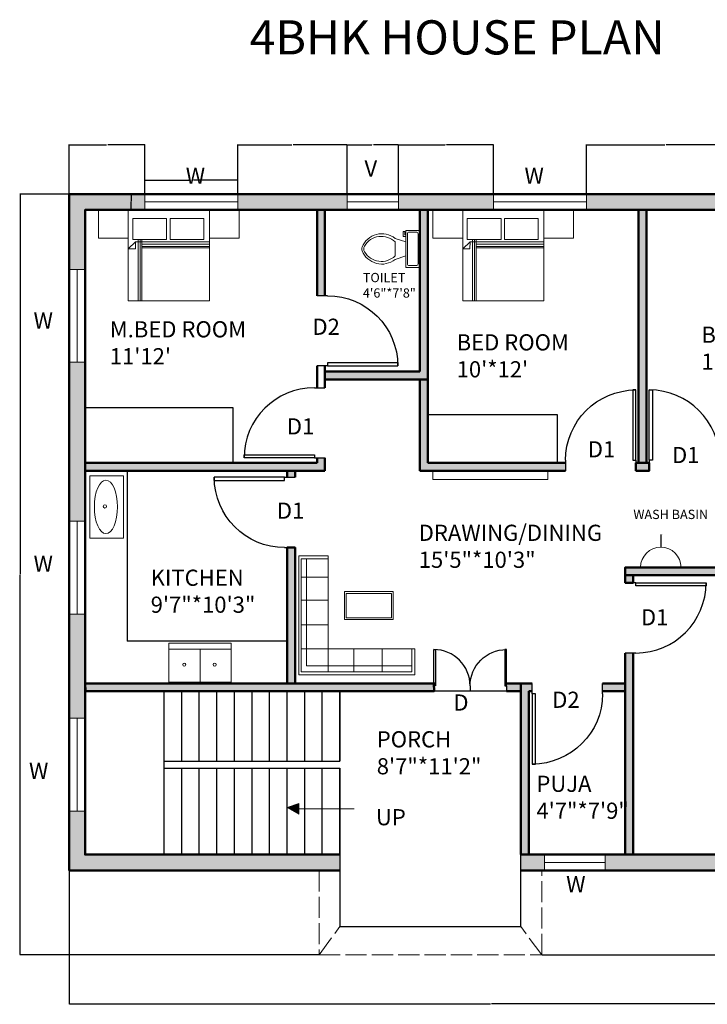
# Model space of a CAD drawing. Units: inches. Extents: x 2116 to 2704, y 2001 to 2561.
# Tile 1 of 2: x 2116 to 2508, y 2001 to 2561. Entities that reach past the tile are written whole.
import ezdxf

# ---------------------------------------------------------------- set-up
doc = ezdxf.new("R2010")
doc.units = ezdxf.units.IN
doc.linetypes.add('ACAD_ISO02W100', pattern=[15, 12, -3])
for name, color, linetype, lineweight in [('A-ANNO-DIMS', 2, 'Continuous', 18), ('A-ANNO-SYMB', 70, 'Continuous', 18), ('A-ANNO-TITL', 7, 'Continuous', 35), ('A-AREA-IDEN', 70, 'Continuous', 25), ('A-DOOR', 3, 'Continuous', 25), ('A-FLOR', 7, 'Continuous', 30), ('A-FLOR-CASE', 9, 'Continuous', 25), ('A-FLOR-FIXT', 9, 'Continuous', 18), ('A-FLOR-OVHD', 8, 'ACAD_ISO02W100', 18), ('A-FLOR-STRS', 7, 'Continuous', 25), ('A-FURN', 40, 'Continuous', 18), ('A-GLAZ', 4, 'Continuous', 20), ('A-WALL-PATT', 172, 'Continuous', 13), ('SINK', 240, 'Continuous', 18), ('TEXT', 70, 'Continuous', 18), ('TV', 210, 'Continuous', 18), ('WALL', 7, 'Continuous', 50)]:
    doc.layers.add(name, color=color, linetype=linetype, lineweight=lineweight)
doc.styles.get("Standard").update_dxf_attribs({"font": 'arial.ttf'})
doc.dimstyles.get("Standard").update_dxf_attribs({"dimtxt": 0.18, "dimasz": 0.18, "dimexe": 0.18, "dimexo": 0.0625, "dimgap": 0.09, "dimtad": 0, "dimtih": 1, "dimtoh": 1, "dimdec": 4, "dimzin": 0, "dimdsep": 46, "dimtxsty": 'Standard', "dimcen": 0.09, "dimadec": 0, "dimazin": 0, "dimtfac": 1, "dimtdec": 4, "dimtofl": 0, "dimtmove": 0, "dimatfit": 3, "dimfxl": 1, "dimtolj": 1, "dimtzin": 0, "dimarcsym": 0})

# ---------------------------------------------------------------- blocks, each defined once
blk = doc.blocks.new('*U2')
for p, q in [((0, 0), (0, -6)), ((40, 0), (40, -6))]:
    blk.add_line(p, q)
blk.add_lwpolyline([(0, 0), (0, 40), (1.75, 40), (1.75, 0)], close=True)
blk.add_arc((0, 0), 40, 0, 90)
blk = doc.blocks.new('*U4')
for p, q in [((9.5, -6), (9.5, -2)), ((-10, -8.5), (-8, -8.5)), ((-10, -9.5), (-10, -8.5)), ((-7, -9.5), (-10, -9.5)), ((-8, -8.5), (-8, -8)), ((-7, -8), (-7, -9.5)), ((-4, -8), (-6, -14)), ((4, -8), (6, -14)), ((4, -14), (-4, -14))]:
    blk.add_line(p, q)
blk.add_lwpolyline([(10.5, -8), (10.5, 0), (-10.5, 0), (-10.5, -8)], close=True)
for points in [[(-9.5, -2), (-9.5, -6)], [(8.5, -1), (-8.5, -1)], [(-8.5, -7), (8.5, -7)]]:
    blk.add_lwpolyline(points)
for centre, radius, start, end in [((-8.62, -1.88), 0.884, 81.8699, 188.1301), ((8.62, -1.88), 0.884, 351.8699, 98.1301), ((-8.62, -6.12), 0.884, 171.8699, 278.1301), ((8.62, -6.12), 0.884, 261.8699, 8.1301), ((3.52, -21.58), 12.17, 141.4691, 247.9714), ((4.2, -21.82), 11.33, 136.3677, 238.9468), ((-3.52, -21.58), 12.17, 292.0284, 38.5307), ((-4.2, -21.82), 11.33, 301.053, 43.6321), ((0, -27.88), 4, 245.7318, 294.2682), ((0, -29), 4, 254.8605, 285.1395)]:
    blk.add_arc(centre, radius, start, end)
blk = doc.blocks.new('BED-DOUBLE-WITH-NIGHTSTANDS')
for p, q in [((22.66, 34.94), (22.66, 0)), ((23.77, 34.94), (23.77, 0)), ((24.74, 34.94), (24.74, 0)), ((21.16, 33.51), (16.99, 29.58)), ((16.99, 29.58), (21.04, 29.58)), ((21.04, 29.58), (21.16, 33.51)), ((63.16, 33.51), (21.16, 33.51)), ((24.74, 32.21), (63.16, 32.21)), ((24.74, 30.97), (63.16, 30.97)), ((24.74, 30.05), (63.16, 30.05))]:
    blk.add_line(p, q)
for points in [[(16.99, 51.74), (0, 51.74), (0, 35.55), (16.99, 35.55)], [(16.99, 51.74), (63.16, 51.74), (63.16, 0), (16.99, 0)], [(80.15, 51.74), (63.16, 51.74), (63.16, 35.55), (80.15, 35.55)], [(19.62, 46.86), (38.84, 46.86), (38.84, 34.94), (19.62, 34.94)], [(40.77, 46.86), (59.99, 46.86), (59.99, 34.94), (40.77, 34.94)]]:
    blk.add_lwpolyline(points, close=True)
blk = doc.blocks.new('WIN-PLAN-53IN-NOM')
blk.add_line((0, 4.5), (52.88, 4.5))
blk.add_lwpolyline([(0, 9), (52.88, 9), (52.88, 0), (0, 0)], close=True)
blk = doc.blocks.new('*D7')
at = {"layer": 'A-ANNO-DIMS', "color": 0, "lineweight": -2, "transparency": 16777216}
for p, q in [((2187.79, 2462.31), (2187.79, 2470.36)), ((2187.97, 2470.18), (2213.11, 2470.18)), ((2240.48, 2470.18), (2215.34, 2470.18)), ((2240.66, 2462.31), (2240.66, 2470.36))]:
    blk.add_line(p, q, dxfattribs=at)
at = {"layer": 'A-ANNO-DIMS', "color": 0, "lineweight": 100, "transparency": 16777216}
for points in [[(2187.97, 2470.21), (2187.97, 2470.15), (2187.79, 2470.18)], [(2240.48, 2470.21), (2240.48, 2470.15), (2240.66, 2470.18)]]:
    blk.add_solid(points, dxfattribs=at)
at = {"layer": 'Defpoints', "color": 0, "lineweight": 100, "transparency": 16777216}
for p in [(2240.66, 2470.18), (2187.79, 2462.24), (2240.66, 2462.24)]:
    blk.add_point(p, dxfattribs=at)
at = {"layer": 'A-ANNO-DIMS', "color": 0, "transparency": 16777216, "insert": (2214.22, 2470.18), "char_height": 0.18, "attachment_point": 5}
blk.add_mtext('\\A1;WINDOW 53 TYP.', dxfattribs=at)
blk = doc.blocks.new('*D8')
at = {"layer": 'A-ANNO-DIMS', "color": 0, "lineweight": -2, "transparency": 16777216}
for p, q in [((2187.72, 2462.24), (2179.67, 2462.24)), ((2179.85, 2462.06), (2179.85, 2457.93)), ((2179.85, 2453.42), (2179.85, 2457.56)), ((2187.72, 2453.24), (2179.67, 2453.24))]:
    blk.add_line(p, q, dxfattribs=at)
at = {"layer": 'A-ANNO-DIMS', "color": 0, "lineweight": 100, "transparency": 16777216}
for points in [[(2179.82, 2462.06), (2179.88, 2462.06), (2179.85, 2462.24)], [(2179.82, 2453.42), (2179.88, 2453.42), (2179.85, 2453.24)]]:
    blk.add_solid(points, dxfattribs=at)
at = {"layer": 'Defpoints', "color": 0, "lineweight": 100, "transparency": 16777216}
for p in [(2179.85, 2462.24), (2187.79, 2462.24), (2187.79, 2453.24)]:
    blk.add_point(p, dxfattribs=at)
at = {"layer": 'A-ANNO-DIMS', "color": 0, "transparency": 16777216, "insert": (2179.85, 2457.74), "char_height": 0.18, "attachment_point": 5}
blk.add_mtext('\\A1;9 TYP.', dxfattribs=at)
blk = doc.blocks.new('*D11')
at = {"layer": 'A-ANNO-DIMS', "color": 0, "lineweight": -2, "transparency": 16777216}
for p, q in [((2144.72, 2462.31), (2144.72, 2490.37)), ((2144.9, 2490.19), (2165.86, 2490.19)), ((2187.61, 2490.19), (2166.65, 2490.19)), ((2187.79, 2462.31), (2187.79, 2490.37))]:
    blk.add_line(p, q, dxfattribs=at)
at = {"layer": 'A-ANNO-DIMS', "color": 0, "lineweight": 100, "transparency": 16777216}
for points in [[(2144.9, 2490.22), (2144.9, 2490.16), (2144.72, 2490.19)], [(2187.61, 2490.22), (2187.61, 2490.16), (2187.79, 2490.19)]]:
    blk.add_solid(points, dxfattribs=at)
at = {"layer": 'Defpoints', "color": 0, "lineweight": 100, "transparency": 16777216}
for p in [(2187.79, 2490.19), (2144.72, 2462.24), (2187.79, 2462.24)]:
    blk.add_point(p, dxfattribs=at)
at = {"layer": 'A-ANNO-DIMS', "color": 0, "transparency": 16777216, "insert": (2166.25, 2490.19), "char_height": 0.18, "attachment_point": 5}
blk.add_mtext('\\A1;43.06', dxfattribs=at)
blk = doc.blocks.new('*D12')
at = {"layer": 'A-ANNO-DIMS', "color": 0, "lineweight": -2, "transparency": 16777216}
for p, q in [((2240.66, 2462.31), (2240.66, 2490.37)), ((2240.84, 2490.19), (2271.39, 2490.19)), ((2302.73, 2490.19), (2272.18, 2490.19)), ((2302.91, 2462.31), (2302.91, 2490.37))]:
    blk.add_line(p, q, dxfattribs=at)
at = {"layer": 'A-ANNO-DIMS', "color": 0, "lineweight": 100, "transparency": 16777216}
for points in [[(2240.84, 2490.22), (2240.84, 2490.16), (2240.66, 2490.19)], [(2302.73, 2490.22), (2302.73, 2490.16), (2302.91, 2490.19)]]:
    blk.add_solid(points, dxfattribs=at)
at = {"layer": 'Defpoints', "color": 0, "lineweight": 100, "transparency": 16777216}
for p in [(2302.91, 2490.19), (2240.66, 2462.24), (2302.91, 2462.24)]:
    blk.add_point(p, dxfattribs=at)
at = {"layer": 'A-ANNO-DIMS', "color": 0, "transparency": 16777216, "insert": (2271.79, 2490.19), "char_height": 0.18, "attachment_point": 5}
blk.add_mtext('\\A1;62.25', dxfattribs=at)
blk = doc.blocks.new('*D13')
at = {"layer": 'A-ANNO-DIMS', "color": 0, "lineweight": -2, "transparency": 16777216}
for p, q in [((2302.91, 2462.31), (2302.91, 2490.37)), ((2303.09, 2490.19), (2317.01, 2490.19)), ((2331.86, 2490.19), (2317.94, 2490.19)), ((2332.04, 2462.31), (2332.04, 2490.37))]:
    blk.add_line(p, q, dxfattribs=at)
at = {"layer": 'A-ANNO-DIMS', "color": 0, "lineweight": 100, "transparency": 16777216}
for points in [[(2303.09, 2490.22), (2303.09, 2490.16), (2302.91, 2490.19)], [(2331.86, 2490.22), (2331.86, 2490.16), (2332.04, 2490.19)]]:
    blk.add_solid(points, dxfattribs=at)
at = {"layer": 'Defpoints', "color": 0, "lineweight": 100, "transparency": 16777216}
for p in [(2332.04, 2490.19), (2302.91, 2462.24), (2332.04, 2462.24)]:
    blk.add_point(p, dxfattribs=at)
at = {"layer": 'A-ANNO-DIMS', "color": 0, "transparency": 16777216, "insert": (2317.47, 2490.19), "char_height": 0.18, "attachment_point": 5}
blk.add_mtext('\\A1;29.126', dxfattribs=at)
blk = doc.blocks.new('*D14')
at = {"layer": 'A-ANNO-DIMS', "color": 0, "lineweight": -2, "transparency": 16777216}
for p, q in [((2332.04, 2462.31), (2332.04, 2490.37)), ((2332.22, 2490.19), (2358.74, 2490.19)), ((2386.04, 2490.19), (2359.52, 2490.19)), ((2386.22, 2462.31), (2386.22, 2490.37))]:
    blk.add_line(p, q, dxfattribs=at)
at = {"layer": 'A-ANNO-DIMS', "color": 0, "lineweight": 100, "transparency": 16777216}
for points in [[(2332.22, 2490.22), (2332.22, 2490.16), (2332.04, 2490.19)], [(2386.04, 2490.22), (2386.04, 2490.16), (2386.22, 2490.19)]]:
    blk.add_solid(points, dxfattribs=at)
at = {"layer": 'Defpoints', "color": 0, "lineweight": 100, "transparency": 16777216}
for p in [(2386.22, 2490.19), (2332.04, 2462.24), (2386.22, 2462.24)]:
    blk.add_point(p, dxfattribs=at)
at = {"layer": 'A-ANNO-DIMS', "color": 0, "transparency": 16777216, "insert": (2359.13, 2490.19), "char_height": 0.18, "attachment_point": 5}
blk.add_mtext('\\A1;54.18', dxfattribs=at)
blk = doc.blocks.new('*D15')
at = {"layer": 'A-ANNO-DIMS', "color": 0, "lineweight": -2, "transparency": 16777216}
for p, q in [((2439.1, 2462.31), (2439.1, 2490.37)), ((2439.28, 2490.19), (2483.65, 2490.19)), ((2528.8, 2490.19), (2484.43, 2490.19)), ((2528.98, 2462.31), (2528.98, 2490.37))]:
    blk.add_line(p, q, dxfattribs=at)
at = {"layer": 'A-ANNO-DIMS', "color": 0, "lineweight": 100, "transparency": 16777216}
for points in [[(2439.28, 2490.22), (2439.28, 2490.16), (2439.1, 2490.19)], [(2528.8, 2490.22), (2528.8, 2490.16), (2528.98, 2490.19)]]:
    blk.add_solid(points, dxfattribs=at)
at = {"layer": 'Defpoints', "color": 0, "lineweight": 100, "transparency": 16777216}
for p in [(2528.98, 2490.19), (2439.1, 2462.24), (2528.98, 2462.24)]:
    blk.add_point(p, dxfattribs=at)
at = {"layer": 'A-ANNO-DIMS', "color": 0, "transparency": 16777216, "insert": (2484.04, 2490.19), "char_height": 0.18, "attachment_point": 5}
blk.add_mtext('\\A1;89.88', dxfattribs=at)
blk = doc.blocks.new('*D16')
at = {"layer": 'A-ANNO-DIMS', "color": 0, "lineweight": -2, "transparency": 16777216}
for p, q in [((2144.72, 2077.18), (2144.72, 2001.04)), ((2624.72, 2077.18), (2624.72, 2001.04)), ((2144.9, 2001.22), (2384.43, 2001.22)), ((2624.54, 2001.22), (2385.01, 2001.22))]:
    blk.add_line(p, q, dxfattribs=at)
at = {"layer": 'A-ANNO-DIMS', "color": 0, "lineweight": 100, "transparency": 16777216}
for points in [[(2144.9, 2001.25), (2144.9, 2001.19), (2144.72, 2001.22)], [(2624.54, 2001.25), (2624.54, 2001.19), (2624.72, 2001.22)]]:
    blk.add_solid(points, dxfattribs=at)
at = {"layer": 'Defpoints', "color": 0, "lineweight": 100, "transparency": 16777216}
for p in [(2144.72, 2077.24), (2624.72, 2077.24), (2624.72, 2001.22)]:
    blk.add_point(p, dxfattribs=at)
at = {"layer": 'A-ANNO-DIMS', "color": 0, "transparency": 16777216, "insert": (2384.72, 2001.22), "char_height": 0.18, "attachment_point": 5}
blk.add_mtext('\\A1;480', dxfattribs=at)
blk = doc.blocks.new('*D21')
at = {"layer": 'A-ANNO-DIMS', "color": 0, "lineweight": -2, "transparency": 16777216}
for p, q in [((2624.78, 2077.24), (2703.85, 2077.24)), ((2703.67, 2077.06), (2703.67, 2053.39)), ((2703.67, 2029.35), (2703.67, 2053.03)), ((2413.8, 2029.17), (2703.85, 2029.17))]:
    blk.add_line(p, q, dxfattribs=at)
at = {"layer": 'A-ANNO-DIMS', "color": 0, "lineweight": 100, "transparency": 16777216}
for points in [[(2703.64, 2077.06), (2703.7, 2077.06), (2703.67, 2077.24)], [(2703.64, 2029.35), (2703.7, 2029.35), (2703.67, 2029.17)]]:
    blk.add_solid(points, dxfattribs=at)
at = {"layer": 'Defpoints', "color": 0, "lineweight": 100, "transparency": 16777216}
for p in [(2624.72, 2077.24), (2703.67, 2077.24), (2413.74, 2029.17)]:
    blk.add_point(p, dxfattribs=at)
at = {"layer": 'A-ANNO-DIMS', "color": 0, "transparency": 16777216, "insert": (2703.67, 2053.21), "char_height": 0.18, "attachment_point": 5}
blk.add_mtext('\\A1;48.07', dxfattribs=at)
blk = doc.blocks.new('*D22')
at = {"layer": 'A-ANNO-DIMS', "color": 0, "lineweight": -2, "transparency": 16777216}
for p, q in [((2144.66, 2462.24), (2116.59, 2462.24)), ((2116.77, 2462.06), (2116.77, 2245.89)), ((2116.77, 2029.35), (2116.77, 2245.53)), ((2286.92, 2029.17), (2116.59, 2029.17))]:
    blk.add_line(p, q, dxfattribs=at)
at = {"layer": 'A-ANNO-DIMS', "color": 0, "lineweight": 100, "transparency": 16777216}
for points in [[(2116.74, 2462.06), (2116.8, 2462.06), (2116.77, 2462.24)], [(2116.74, 2029.35), (2116.8, 2029.35), (2116.77, 2029.17)]]:
    blk.add_solid(points, dxfattribs=at)
at = {"layer": 'Defpoints', "color": 0, "lineweight": 100, "transparency": 16777216}
for p in [(2116.77, 2462.24), (2144.72, 2462.24), (2286.98, 2029.17)]:
    blk.add_point(p, dxfattribs=at)
at = {"layer": 'A-ANNO-DIMS', "color": 0, "transparency": 16777216, "insert": (2116.77, 2245.71), "char_height": 0.18, "attachment_point": 5}
blk.add_mtext('\\A1;433.1', dxfattribs=at)
blk = doc.blocks.new('*D23')
at = {"layer": 'A-ANNO-DIMS', "color": 0, "lineweight": -2, "transparency": 16777216}
for p, q in [((2481.6, 2268.18), (2481.42, 2268.18)), ((2481.42, 2268.18), (2481.42, 2261.45)), ((2481.33, 2249.74), (2481.51, 2249.74)), ((2481.42, 2249.65), (2481.42, 2249.83))]:
    blk.add_line(p, q, dxfattribs=at)
at = {"layer": 'A-ANNO-DIMS', "color": 0, "lineweight": 100, "transparency": 16777216}
blk.add_solid([(2481.39, 2261.45), (2481.45, 2261.45), (2481.42, 2261.27)], dxfattribs=at)
at = {"layer": 'Defpoints', "color": 0, "lineweight": 100, "transparency": 16777216}
for p in [(2481.42, 2261.27), (2481.42, 2249.74)]:
    blk.add_point(p, dxfattribs=at)
at = {"layer": 'A-ANNO-DIMS', "color": 0, "transparency": 16777216, "insert": (2482.15, 2268.18), "char_height": 0.18, "attachment_point": 5}
blk.add_mtext('\\A1;R11.525', dxfattribs=at)

msp = doc.modelspace()

# ---------------------------------------------------------------- hatches: boundary and pattern name
at = {"layer": 'A-ANNO-SYMB'}
h = msp.add_hatch(color=256, dxfattribs=at)
h.dxf.hatch_style = 1
h.paths.add_polyline_path([(2275.4473, 2115.2764), (2268.722, 2113.1221), (2275.4473, 2109.2764), (2275.4473, 2112.2764)])
at = {"layer": 'A-WALL-PATT'}
h = msp.add_hatch(color=256, dxfattribs=at)
h.dxf.hatch_style = 1
h.paths.add_polyline_path([(2187.7856, 2462.2434), (2144.722, 2462.2434), (2144.722, 2419.3525), (2153.722, 2419.3525), (2153.722, 2453.2434), (2187.7856, 2453.2434)])
h.paths.add_polyline_path([(2302.9116, 2462.2434), (2240.6643, 2462.2434), (2240.6643, 2453.2434), (2241.4366, 2453.2434), (2285.722, 2453.2434), (2302.9116, 2453.2434)])
h.paths.add_polyline_path([(2153.722, 2366.4738), (2144.722, 2366.4738), (2144.722, 2275.9883), (2153.722, 2275.9883)])
h.paths.add_polyline_path([(2386.2219, 2462.2434), (2332.038, 2462.2434), (2332.038, 2453.2434), (2344.222, 2453.2434), (2386.2219, 2453.2434)])
h.paths.add_polyline_path([(2528.9791, 2462.2434), (2439.1006, 2462.2434), (2439.1006, 2453.2434), (2528.9791, 2453.2434)])
h.paths.add_polyline_path([(2624.722, 2462.2434), (2581.8578, 2462.2434), (2581.8578, 2453.2434), (2594.0001, 2453.2434), (2610.9949, 2453.2434), (2615.722, 2453.2434), (2615.722, 2415.194), (2624.722, 2415.194)])
h = msp.add_hatch(color=256, dxfattribs=at)
h.dxf.hatch_style = 1
h.paths.add_polyline_path([(2473.222, 2453.2434), (2468.722, 2453.2434), (2468.722, 2309.2434), (2473.222, 2309.2434)])
h.paths.add_polyline_path([(2474.8589, 2309.2434), (2467.2113, 2309.2434), (2467.2113, 2304.7434), (2474.8589, 2304.7434)])
h.paths.add_polyline_path([(2615.722, 2309.2434), (2514.8589, 2309.2434), (2514.8589, 2304.7434), (2615.722, 2304.7434)])
h.paths.add_polyline_path([(2624.722, 2362.3153), (2615.722, 2362.3153), (2615.722, 2309.2434), (2615.722, 2304.7434), (2615.722, 2291.4101), (2624.722, 2291.4101)])
h.paths.add_polyline_path([(2348.722, 2336.7395), (2348.722, 2356.7434), (2344.222, 2356.7434), (2344.222, 2304.7434), (2427.2113, 2304.7434), (2427.2113, 2309.2434), (2348.722, 2309.2434)])
h.paths.add_polyline_path([(2348.722, 2453.2434), (2344.222, 2453.2434), (2344.222, 2361.2434), (2290.222, 2361.2434), (2290.222, 2356.7434), (2348.722, 2356.7434)])
h.paths.add_polyline_path([(2290.222, 2453.2434), (2285.722, 2453.2434), (2285.722, 2404.3805), (2290.222, 2404.3805)])
h.paths.add_polyline_path([(2290.222, 2312.0296), (2285.722, 2312.0296), (2285.722, 2309.2434), (2153.722, 2309.2434), (2153.722, 2304.7434), (2177.722, 2304.7434), (2268.722, 2304.7434), (2290.222, 2304.7434)])
h.paths.add_polyline_path([(2273.222, 2304.7434), (2268.722, 2304.7434), (2268.722, 2301.0301), (2273.222, 2301.0301)])
h = msp.add_hatch(color=256, dxfattribs=at)
h.dxf.hatch_style = 1
h.paths.add_polyline_path([(2406.222, 2179.2434), (2408.2564, 2179.2434), (2408.2564, 2183.7434), (2401.722, 2183.7434), (2401.722, 2086.2434), (2406.222, 2086.2434)])
h.paths.add_polyline_path([(2465.722, 2200.9957), (2461.222, 2200.9957), (2461.222, 2086.2434), (2465.722, 2086.2434)])
h.paths.add_polyline_path([(2461.222, 2183.7434), (2448.2564, 2183.7434), (2448.2564, 2179.2434), (2461.222, 2179.2434)])
h.paths.add_polyline_path([(2401.722, 2183.7434), (2393.523, 2183.7434), (2393.523, 2182.34), (2393.523, 2179.2434), (2401.722, 2179.2434)])
h.paths.add_polyline_path([(2415.304, 2086.2434), (2406.222, 2086.2434), (2401.722, 2086.2434), (2401.722, 2077.2434), (2415.304, 2077.2434)])
h.paths.add_polyline_path([(2298.722, 2086.2434), (2153.722, 2086.2434), (2153.722, 2111.0387), (2144.722, 2111.0387), (2144.722, 2077.2434), (2298.722, 2077.2434)])
h.paths.add_polyline_path([(2360.0446, 2163.1907), (2373.9305, 2163.1907), (2373.9305, 2182.1552), (2360.0446, 2182.1552)], flags=9)
h.paths.add_polyline_path([(2315.961, 2097.9087), (2338.4221, 2097.9087), (2338.4221, 2116.8732), (2315.961, 2116.8732)], flags=9)
h.paths.add_polyline_path([(2316.4397, 2126.7155), (2376.3025, 2126.7155), (2376.3025, 2161.0558), (2316.4397, 2161.0558)], flags=9)
h.paths.add_polyline_path([(2521.5838, 2259.7103), (2542.6199, 2259.7103), (2542.6199, 2278.6748), (2521.5838, 2278.6748)], flags=9)
h.paths.add_polyline_path([(2484.5309, 2304.0263), (2505.567, 2304.0263), (2505.567, 2322.9908), (2484.5309, 2322.9908)], flags=9)
h.paths.add_polyline_path([(2436.5934, 2307.3012), (2457.6295, 2307.3012), (2457.6295, 2326.2657), (2436.5934, 2326.2657)], flags=9)
h.paths.add_polyline_path([(2279.8188, 2377.038), (2300.8549, 2377.038), (2300.8549, 2396.0025), (2279.8188, 2396.0025)], flags=9)
h.paths.add_polyline_path([(2265.2604, 2320.3349), (2286.2965, 2320.3349), (2286.2965, 2339.2994), (2265.2604, 2339.2994)], flags=9)
h.paths.add_polyline_path([(2259.5917, 2272.3677), (2280.6278, 2272.3677), (2280.6278, 2291.3322), (2259.5917, 2291.3322)], flags=9)
h.paths.add_polyline_path([(2466.8383, 2211.6782), (2487.8744, 2211.6782), (2487.8744, 2230.6428), (2466.8383, 2230.6428)], flags=9)
h.paths.add_polyline_path([(2416.3041, 2164.7232), (2437.3402, 2164.7232), (2437.3402, 2183.6877), (2416.3041, 2183.6877)], flags=9)
h.paths.add_polyline_path([(2464.3943, 2274.2881), (2513.2984, 2274.2881), (2513.2984, 2285.1577), (2464.3943, 2285.1577)], flags=9)
h.paths.add_polyline_path([(2558.3191, 2283.0075), (2588.2617, 2283.0075), (2588.2617, 2302.6898), (2558.3191, 2302.6898)], flags=9)
h.paths.add_polyline_path([(2187.7928, 2218.693), (2248.8232, 2218.693), (2248.8232, 2253.0333), (2187.7928, 2253.0333)], flags=9)
h.paths.add_polyline_path([(2407.3216, 2101.5621), (2460.3921, 2101.5621), (2460.3921, 2135.9024), (2407.3216, 2135.9024)], flags=9)
h.paths.add_polyline_path([(2516.1575, 2162.0461), (2609.3291, 2162.0461), (2609.3291, 2196.3865), (2516.1575, 2196.3865)], flags=9)
h.paths.add_polyline_path([(2339.9087, 2244.2645), (2455.623, 2244.2645), (2455.623, 2278.6049), (2339.9087, 2278.6049)], flags=9)
h.paths.add_polyline_path([(2500.8533, 2357.0199), (2575.9141, 2357.0199), (2575.9141, 2391.3602), (2500.8533, 2391.3602)], flags=9)
h.paths.add_polyline_path([(2361.5168, 2352.6691), (2436.5776, 2352.6691), (2436.5776, 2387.0094), (2361.5168, 2387.0094)], flags=9)
h.paths.add_polyline_path([(2310.3217, 2400.2918), (2340.3434, 2400.2918), (2340.3434, 2419.9741), (2310.3217, 2419.9741)], flags=9)
h.paths.add_polyline_path([(2164.0511, 2360.101), (2253.3807, 2360.101), (2253.3807, 2394.4413), (2164.0511, 2394.4413)], flags=9)
h = msp.add_hatch(color=256, dxfattribs=at)
h.dxf.hatch_style = 1
h.paths.add_polyline_path([(2624.722, 2150.901), (2615.722, 2150.901), (2615.722, 2086.2434), (2569.9026, 2086.2434), (2569.9026, 2077.2434), (2624.722, 2077.2434)])
h.paths.add_polyline_path([(2517.0239, 2086.2434), (2465.722, 2086.2434), (2449.7631, 2086.2434), (2449.7631, 2077.2434), (2517.0239, 2077.2434)])
h.paths.add_polyline_path([(2624.722, 2262.3456), (2615.722, 2262.3456), (2615.722, 2249.7434), (2615.722, 2203.7797), (2624.722, 2203.7797)])
h.paths.add_polyline_path([(2521.5838, 2259.7103), (2542.6199, 2259.7103), (2542.6199, 2278.6748), (2521.5838, 2278.6748)], flags=9)
h.paths.add_polyline_path([(2484.5309, 2304.0263), (2505.567, 2304.0263), (2505.567, 2322.9908), (2484.5309, 2322.9908)], flags=9)
h.paths.add_polyline_path([(2436.5934, 2307.3012), (2457.6295, 2307.3012), (2457.6295, 2326.2657), (2436.5934, 2326.2657)], flags=9)
h.paths.add_polyline_path([(2279.8188, 2377.038), (2300.8549, 2377.038), (2300.8549, 2396.0025), (2279.8188, 2396.0025)], flags=9)
h.paths.add_polyline_path([(2265.2604, 2320.3349), (2286.2965, 2320.3349), (2286.2965, 2339.2994), (2265.2604, 2339.2994)], flags=9)
h.paths.add_polyline_path([(2259.5917, 2272.3677), (2280.6278, 2272.3677), (2280.6278, 2291.3322), (2259.5917, 2291.3322)], flags=9)
h.paths.add_polyline_path([(2466.8383, 2211.6782), (2487.8744, 2211.6782), (2487.8744, 2230.6428), (2466.8383, 2230.6428)], flags=9)
h.paths.add_polyline_path([(2416.3041, 2164.7232), (2437.3402, 2164.7232), (2437.3402, 2183.6877), (2416.3041, 2183.6877)], flags=9)
h.paths.add_polyline_path([(2464.3943, 2274.2881), (2513.2984, 2274.2881), (2513.2984, 2285.1577), (2464.3943, 2285.1577)], flags=9)
h.paths.add_polyline_path([(2558.3191, 2283.0075), (2588.2617, 2283.0075), (2588.2617, 2302.6898), (2558.3191, 2302.6898)], flags=9)
h.paths.add_polyline_path([(2187.7928, 2218.693), (2248.8232, 2218.693), (2248.8232, 2253.0333), (2187.7928, 2253.0333)], flags=9)
h.paths.add_polyline_path([(2407.3216, 2101.5621), (2460.3921, 2101.5621), (2460.3921, 2135.9024), (2407.3216, 2135.9024)], flags=9)
h.paths.add_polyline_path([(2516.1575, 2162.0461), (2609.3291, 2162.0461), (2609.3291, 2196.3865), (2516.1575, 2196.3865)], flags=9)
h.paths.add_polyline_path([(2339.9087, 2244.2645), (2455.623, 2244.2645), (2455.623, 2278.6049), (2339.9087, 2278.6049)], flags=9)
h.paths.add_polyline_path([(2500.8533, 2357.0199), (2575.9141, 2357.0199), (2575.9141, 2391.3602), (2500.8533, 2391.3602)], flags=9)
h.paths.add_polyline_path([(2361.5168, 2352.6691), (2436.5776, 2352.6691), (2436.5776, 2387.0094), (2361.5168, 2387.0094)], flags=9)
h.paths.add_polyline_path([(2310.3217, 2400.2918), (2340.3434, 2400.2918), (2340.3434, 2419.9741), (2310.3217, 2419.9741)], flags=9)
h.paths.add_polyline_path([(2164.0511, 2360.101), (2253.3807, 2360.101), (2253.3807, 2394.4413), (2164.0511, 2394.4413)], flags=9)
h = msp.add_hatch(color=256, dxfattribs=at)
h.dxf.hatch_style = 1
h.paths.add_polyline_path([(2615.722, 2249.7434), (2461.222, 2249.7434), (2461.222, 2245.3695), (2465.722, 2245.3695), (2615.722, 2245.3695)])
h.paths.add_polyline_path([(2465.722, 2245.3695), (2461.222, 2245.3695), (2461.222, 2240.9957), (2465.722, 2240.9957)])
h.paths.add_polyline_path([(2153.722, 2223.1096), (2144.722, 2223.1096), (2144.722, 2163.9174), (2153.722, 2163.9174)])
h.paths.add_polyline_path([(2352.235, 2183.7434), (2153.722, 2183.7434), (2153.8615, 2179.2434), (2352.235, 2179.2434), (2352.235, 2182.34)])
h.paths.add_polyline_path([(2273.222, 2261.0301), (2268.722, 2261.0301), (2268.722, 2183.7434), (2273.222, 2183.7434)])

# ---------------------------------------------------------------- linework, layer by layer
at = {"layer": 'A-ANNO-SYMB'}
for p, q in [((2268.722, 2113.1221), (2275.4473, 2115.2764)), ((2275.4473, 2109.2764), (2268.722, 2113.1221)), ((2275.4473, 2112.2764), (2275.4473, 2115.2764)), ((2275.4473, 2115.2764), (2275.4473, 2112.2764)), ((2306.9351, 2112.2764), (2275.4473, 2112.2764)), ((2275.4473, 2112.2764), (2275.4473, 2109.2764))]:
    msp.add_line(p, q, dxfattribs=at)
at = {"layer": 'A-FLOR'}
for p, q in [((2401.722, 2179.2434), (2298.722, 2179.2434)), ((2298.722, 2179.2434), (2298.722, 2139.4781)), ((2298.722, 2135.4781), (2298.722, 2045.2434)), ((2401.722, 2045.2434), (2401.722, 2091.9119)), ((2298.722, 2045.2434), (2401.722, 2045.2434))]:
    msp.add_line(p, q, dxfattribs=at)
at = {"layer": 'A-FLOR-CASE'}
for p, q in [((2153.722, 2304.7434), (2177.722, 2304.7434)), ((2177.722, 2304.7434), (2177.722, 2207.7434)), ((2268.722, 2207.7434), (2177.722, 2207.7434)), ((2268.722, 2183.7434), (2268.722, 2207.7434))]:
    msp.add_line(p, q, dxfattribs=at)
for points in [[(2237.8926, 2309.2434), (2153.722, 2309.2434), (2153.722, 2340.7088), (2237.8926, 2340.7088)], [(2422.3599, 2309.2434), (2348.722, 2309.2434), (2348.722, 2336.7395), (2422.3599, 2336.7395)]]:
    msp.add_lwpolyline(points, close=True, dxfattribs=at)
at = {"layer": 'A-FLOR-OVHD'}
for p, q in [((2286.9794, 2077.2434), (2286.9794, 2029.1738)), ((2413.7384, 2029.1738), (2413.7384, 2077.2434)), ((2286.9794, 2029.1738), (2298.722, 2045.2434)), ((2413.7384, 2029.1738), (2401.722, 2045.2434)), ((2286.9794, 2029.1738), (2413.7384, 2029.1738))]:
    msp.add_line(p, q, dxfattribs=at)
at = {"layer": 'A-FLOR-STRS'}
for p, q in [((2198.722, 2086.2434), (2198.722, 2179.2434)), ((2208.722, 2139.4781), (2208.722, 2179.2434)), ((2218.722, 2139.4781), (2218.722, 2179.2434)), ((2228.722, 2139.4781), (2228.722, 2179.2434)), ((2238.722, 2139.4781), (2238.722, 2179.2434)), ((2248.722, 2139.4781), (2248.722, 2179.2434)), ((2258.722, 2139.4781), (2258.722, 2179.2434)), ((2268.722, 2139.4781), (2268.722, 2179.2434)), ((2278.722, 2139.4781), (2278.722, 2179.2434)), ((2288.722, 2139.4781), (2288.722, 2179.2434)), ((2298.722, 2139.4781), (2298.722, 2179.2434)), ((2198.722, 2139.4781), (2298.722, 2139.4781)), ((2198.722, 2135.4781), (2298.722, 2135.4781)), ((2208.722, 2086.2434), (2208.722, 2135.4781)), ((2218.722, 2086.2434), (2218.722, 2135.4781)), ((2228.722, 2086.2434), (2228.722, 2135.4781)), ((2238.722, 2086.2434), (2238.722, 2135.4781)), ((2248.722, 2086.2434), (2248.722, 2135.4781)), ((2258.722, 2086.2434), (2258.722, 2135.4781)), ((2268.722, 2086.2434), (2268.722, 2135.4781)), ((2278.722, 2086.2434), (2278.722, 2135.4781)), ((2288.722, 2086.2434), (2288.722, 2135.4781)), ((2298.722, 2086.2434), (2298.722, 2135.4781))]:
    msp.add_line(p, q, dxfattribs=at)
at = {"layer": 'A-FURN'}
for p, q in [((2292.045, 2256.314), (2275.3699, 2256.314)), ((2275.3699, 2256.314), (2275.3699, 2188.5784)), ((2279.7892, 2254.568), (2279.7892, 2193.6527)), ((2292.045, 2254.568), (2292.045, 2256.314)), ((2276.7505, 2244.2247), (2292.045, 2244.2247)), ((2276.7505, 2231.0108), (2292.045, 2231.0108)), ((2276.7505, 2216.9535), (2292.045, 2216.9535)), ((2306.7242, 2190.293), (2306.7242, 2203.3278)), ((2322.7623, 2190.293), (2322.7623, 2203.3278)), ((2341.3486, 2203.3278), (2339.7275, 2203.3278)), ((2341.3486, 2188.5784), (2341.3486, 2203.3278)), ((2279.7892, 2193.6527), (2339.7275, 2193.6527)), ((2275.3699, 2188.5784), (2341.3486, 2188.5784))]:
    msp.add_line(p, q, dxfattribs=at)
for points in [[(2276.7505, 2190.293), (2292.045, 2190.293), (2292.045, 2254.568), (2276.7505, 2254.568)], [(2301.3629, 2235.9469), (2329.1084, 2235.9469), (2329.1084, 2220.0301), (2301.3629, 2220.0301)], [(2302.3629, 2234.9469), (2328.1084, 2234.9469), (2328.1084, 2221.0301), (2302.3629, 2221.0301)], [(2276.7505, 2190.293), (2339.7275, 2190.293), (2339.7275, 2203.3278), (2276.7505, 2203.3278)]]:
    msp.add_lwpolyline(points, close=True, dxfattribs=at)
at = {"layer": 'A-GLAZ'}
for p, q in [((2302.9116, 2457.7434), (2332.038, 2457.7434)), ((2415.304, 2081.7434), (2449.7631, 2081.7434))]:
    msp.add_line(p, q, dxfattribs=at)
for points in [[(2302.9116, 2453.2434), (2332.038, 2453.2434), (2332.038, 2462.2434), (2302.9116, 2462.2434)], [(2415.304, 2086.2434), (2449.7631, 2086.2434), (2449.7631, 2077.2434), (2415.304, 2077.2434)]]:
    msp.add_lwpolyline(points, close=True, dxfattribs=at)
at = {"layer": 'SINK'}
for p, q in [((2201.3842, 2203.2032), (2236.8447, 2203.2032)), ((2219.1145, 2203.2032), (2219.1145, 2184.481))]:
    msp.add_line(p, q, dxfattribs=at)
for points in [[(2156.3044, 2301.9191), (2175.5956, 2301.9191), (2175.5956, 2266.4404), (2156.3044, 2266.4404)], [(2201.3842, 2206.6152), (2236.8447, 2206.6152), (2236.8447, 2184.481), (2201.3842, 2184.481)]]:
    msp.add_lwpolyline(points, close=True, dxfattribs=at)
for centre, radius in [((2164.9714, 2284.4591), 0.9785), ((2210.1235, 2194.4139), 0.878), ((2227.4406, 2194.4139), 0.878)]:
    msp.add_circle(centre, radius, dxfattribs=at)
msp.add_arc((2481.4217, 2249.7434), 11.5246, 0, 180, dxfattribs=at)
msp.add_ellipse((2165.5306, 2284.1797), major_axis=(0, 15.2251), ratio=0.43153672, dxfattribs=at)
at = {"layer": 'TV'}
msp.add_lwpolyline([(2351.5657, 2304.7434), (2417.0941, 2304.7434), (2417.0941, 2299.8067), (2351.5657, 2299.8067)], close=True, dxfattribs=at)
at = {"layer": 'WALL'}
for p, q in [((2153.722, 2453.2434), (2285.722, 2453.2434)), ((2285.722, 2453.2434), (2285.722, 2404.3805)), ((2290.222, 2453.2434), (2290.222, 2404.3805)), ((2290.222, 2453.2434), (2344.222, 2453.2434)), ((2344.222, 2453.2434), (2344.222, 2361.2434)), ((2348.722, 2453.2434), (2348.722, 2356.7434)), ((2348.722, 2453.2434), (2468.722, 2453.2434)), ((2468.722, 2453.2434), (2468.722, 2309.2434)), ((2473.222, 2453.2434), (2473.222, 2309.2434)), ((2285.722, 2364.3805), (2285.722, 2352.0296)), ((2290.222, 2364.3805), (2290.222, 2352.0296)), ((2344.222, 2361.2434), (2290.222, 2361.2434)), ((2348.722, 2356.7434), (2290.222, 2356.7434)), ((2344.222, 2304.7434), (2344.222, 2356.7434)), ((2348.722, 2309.2434), (2348.722, 2356.7434)), ((2285.722, 2309.2434), (2153.722, 2309.2434)), ((2285.722, 2312.0296), (2285.722, 2309.2434)), ((2290.222, 2312.0296), (2290.222, 2304.7434)), ((2427.2113, 2309.2434), (2348.722, 2309.2434)), ((2468.722, 2309.2434), (2467.2113, 2309.2434)), ((2473.222, 2309.2434), (2474.8589, 2309.2434)), ((2290.222, 2304.7434), (2153.722, 2304.7434)), ((2153.722, 2304.7434), (2268.722, 2304.7434)), ((2268.722, 2304.7434), (2268.722, 2301.0301)), ((2273.222, 2304.7434), (2273.222, 2301.0301)), ((2427.2113, 2304.7434), (2344.222, 2304.7434)), ((2473.222, 2304.7434), (2467.2113, 2304.7434)), ((2473.222, 2304.7434), (2474.8589, 2304.7434)), ((2268.722, 2261.0301), (2268.722, 2183.7434)), ((2273.222, 2261.0301), (2273.222, 2183.7434)), ((2461.222, 2249.7434), (2519.222, 2249.7434)), ((2461.222, 2240.9957), (2461.222, 2249.7434)), ((2465.722, 2242.2434), (2465.722, 2245.2434)), ((2465.722, 2245.2434), (2521.3308, 2245.2434)), ((2465.722, 2240.9957), (2465.722, 2242.2434)), ((2461.222, 2086.2434), (2461.222, 2200.9957)), ((2465.722, 2086.2434), (2465.722, 2200.9957)), ((2353.1382, 2183.7434), (2153.722, 2183.7434)), ((2372.9268, 2183.7434), (2372.8313, 2183.7434)), ((2401.722, 2183.7434), (2392.6198, 2183.7434)), ((2401.722, 2086.2434), (2401.722, 2183.7434)), ((2401.722, 2183.7434), (2408.2564, 2183.7434)), ((2448.2564, 2183.7434), (2461.222, 2183.7434)), ((2352.235, 2179.2434), (2153.722, 2179.2434)), ((2401.722, 2179.2434), (2393.523, 2179.2434)), ((2406.222, 2086.2434), (2406.222, 2179.2434)), ((2406.222, 2179.2434), (2408.2564, 2179.2434)), ((2448.2564, 2179.2434), (2461.222, 2179.2434)), ((2461.222, 2086.2434), (2406.222, 2086.2434)), ((2615.722, 2086.2434), (2465.722, 2086.2434))]:
    msp.add_line(p, q, dxfattribs=at)
for points in [[(2401.722, 2077.2434), (2624.722, 2077.2434), (2624.722, 2462.2434), (2144.722, 2462.2434), (2144.722, 2077.2434), (2298.722, 2077.2434)], [(2615.722, 2309.2434), (2615.722, 2453.2434), (2153.722, 2453.2434), (2153.722, 2086.2434), (2298.722, 2086.2434)], [(2401.722, 2086.2434), (2615.722, 2086.2434), (2615.722, 2304.7434)]]:
    msp.add_lwpolyline(points, dxfattribs=at)
for points in [[(2468.722, 2453.2434), (2473.222, 2453.2434), (2473.222, 2309.2434), (2468.722, 2309.2434)], [(2467.2113, 2304.7434), (2474.8589, 2304.7434), (2474.8589, 2309.2434), (2467.2113, 2309.2434)], [(2268.722, 2183.7434), (2273.222, 2183.7434), (2273.222, 2261.0301), (2268.722, 2261.0301)], [(2615.722, 2249.7434), (2461.222, 2249.7434), (2461.222, 2245.3695), (2615.722, 2245.3695)], [(2461.222, 2245.3695), (2465.722, 2245.3695), (2465.722, 2240.9957), (2461.222, 2240.9957)], [(2153.722, 2183.7434), (2352.235, 2183.7434), (2352.3746, 2179.2434), (2153.8615, 2179.2434)]]:
    msp.add_lwpolyline(points, close=True, dxfattribs=at)

# ---------------------------------------------------------------- block references
at = {"layer": 'A-DOOR', "xscale": -1}
for p, rotation in [((2291.722, 2364.3805), 270), ((2267.222, 2301.0301), 90), ((2408.2564, 2177.7434), 180)]:
    msp.add_blockref('*U2', p, dxfattribs=dict(at, rotation=rotation))
at = {"layer": 'A-DOOR'}
for p, rotation in [((2284.222, 2312.0296), 90), ((2467.222, 2240.9957), 270)]:
    msp.add_blockref('*U2', p, dxfattribs=dict(at, rotation=rotation))
at = {"layer": 'A-DOOR', "xscale": -1}
msp.add_blockref('*U2', (2467.2113, 2310.7434), dxfattribs=at)
at = {"layer": 'A-DOOR'}
msp.add_blockref('*U2', (2474.8589, 2310.7434), dxfattribs=at)
at = {"layer": 'A-DOOR', "yscale": 0.5160995705010885, "zscale": 0.5160995705010885}
for p, xscale in [((2352.235, 2182.34), 0.5160995705010885), ((2393.523, 2182.34), -0.5160995705010885)]:
    msp.add_blockref('*U2', p, dxfattribs=dict(at, xscale=xscale))
at = {"layer": 'A-FLOR-FIXT', "rotation": 270}
msp.add_blockref('*U4', (2344.222, 2431.0232), dxfattribs=at)
at = {"layer": 'A-FURN'}
for p in [(2161.2831, 2401.5064), (2351.6488, 2401.5064)]:
    msp.add_blockref('BED-DOUBLE-WITH-NIGHTSTANDS', p, dxfattribs=at)
at = {"layer": 'A-GLAZ'}
for p in [(2187.7856, 2453.2434), (2386.2219, 2453.2434)]:
    msp.add_blockref('WIN-PLAN-53IN-NOM', p, dxfattribs=at)
at = {"layer": 'A-GLAZ', "rotation": 270.0000000000007}
for p in [(2144.722, 2419.3525), (2144.722, 2275.9883), (2144.722, 2163.9174)]:
    msp.add_blockref('WIN-PLAN-53IN-NOM', p, dxfattribs=at)

# ---------------------------------------------------------------- texts
at = {"layer": 'A-ANNO-TITL', "insert": (2247.3512, 2561.1454), "char_height": 19.42881, "attachment_point": 1}
msp.add_mtext_dynamic_manual_height_columns('4BHK HOUSE PLAN', width=1490.040939, gutter_width=97.144, heights=[0], dxfattribs=at)
at = {"layer": 'A-AREA-IDEN', "attachment_point": 1}
for s, width, gutter_width, insert, char_height in [('TOILET\\P4\'6"*7\'8"', 168.791536, 26.3734, (2311.813, 2417.353), 5.27468), ("M.BED ROOM\\P11'12'", 294.496073, 46.0145, (2167.7517, 2389.8681), 9.2029), ("BED ROOM\\P10'*12'", 294.496073, 46.0145, (2365.2175, 2382.4362), 9.2029), ('BED ROOM\\P11\'7"*12\'', 294.496073, 46.0145, (2504.5539, 2386.787), 9.2029), ('DRAWING/DINING\\P15\'5"*10\'3"', 294.496073, 46.0145, (2343.6093, 2274.0254), 9.202903), ('KITCHEN\\P9\'7"*10\'3"', 294.496073, 46.0145, (2191.0351, 2248.4538), 9.2029), ('PORCH\\P8\'7"*11\'2"', 294.496073, 46.0145, (2319.7323, 2156.4826), 9.2029), ('PUJA\\P4\'7"*7\'9"', 294.496073, 46.0145, (2410.6142, 2131.166), 9.2029)]:
    msp.add_mtext_dynamic_manual_height_columns(s, width=width, gutter_width=gutter_width, heights=[0], dxfattribs=dict(at, insert=insert, char_height=char_height))
at = {"layer": 'TEXT', "attachment_point": 1}
for s, width, gutter_width, insert, char_height in [('W', 294.496073, 46.0145, (2210.9909, 2477.3001), 9.2029), ('V', 294.496073, 46.0145, (2312.7303, 2481.4373), 9.2029), ('W', 294.496073, 46.0145, (2403.8225, 2477.3001), 9.2029), ('W', 294.496073, 46.0145, (2124.3637, 2394.8269), 9.2029), ('D2', 294.496073, 46.0145, (2283.1114, 2391.3037), 9.2029), ('D1', 294.496073, 46.0145, (2268.553, 2334.6007), 9.2029), ('D1', 294.496073, 46.0145, (2439.886, 2321.5669), 9.2029), ('D1', 294.496073, 46.0145, (2487.8235, 2318.292), 9.2029), ('D1', 294.496073, 46.0145, (2262.8843, 2286.6335), 9.2029), ('WASH BASIN', 168.791536, 26.3734, (2465.8029, 2282.5329), 5.27468), ('W', 294.496073, 46.0145, (2124.3637, 2256.432), 9.2029), ('D1', 294.496073, 46.0145, (2470.1308, 2225.944), 9.2029), ('D', 294.496073, 46.0145, (2363.3372, 2177.4188), 9.2029), ('D2', 294.496073, 46.0145, (2419.5966, 2178.989), 9.2029), ('W', 294.496073, 46.0145, (2121.7669, 2138.5282), 9.2029), ('UP', 294.496073, 46.0145, (2319.2724, 2112.1368), 9.2029), ('W', 294.496073, 46.0145, (2427.5534, 2073.9921), 9.2029)]:
    msp.add_mtext_dynamic_manual_height_columns(s, width=width, gutter_width=gutter_width, heights=[0], dxfattribs=dict(at, insert=insert, char_height=char_height))

# ---------------------------------------------------------------- dimensions: what is measured, and where the dimension line sits
at = {"layer": 'A-ANNO-DIMS'}
for base, p1, p2, override, picture, middle in [((2187.7856, 2490.1934), (2144.722, 2462.2434), (2187.7856, 2462.2434), {"dimdec": 2, "dimlfac": 1, "dimrnd": 0, "dimzin": 0, "dimdsep": 46, "dimlunit": 2}, '*D11', (2166.2538, 2490.1934)), ((2302.9116, 2490.1934), (2240.6643, 2462.2434), (2302.9116, 2462.2434), {"dimdec": 2, "dimlfac": 1, "dimrnd": 0, "dimzin": 0, "dimdsep": 46, "dimlunit": 2}, '*D12', (2271.788, 2490.1934)), ((2332.038, 2490.1934), (2302.9116, 2462.2434), (2332.038, 2462.2434), {"dimdec": 3, "dimlfac": 1, "dimrnd": 0, "dimzin": 0, "dimdsep": 46, "dimlunit": 2}, '*D13', (2317.4748, 2490.1934)), ((2386.2219, 2490.1934), (2332.038, 2462.2434), (2386.2219, 2462.2434), {"dimdec": 2, "dimlfac": 1, "dimrnd": 0, "dimzin": 0, "dimdsep": 46, "dimlunit": 2}, '*D14', (2359.13, 2490.1934)), ((2528.9791, 2490.1934), (2439.1006, 2462.2434), (2528.9791, 2462.2434), {"dimdec": 2, "dimlfac": 1, "dimrnd": 0, "dimzin": 0, "dimdsep": 46, "dimlunit": 2}, '*D15', (2484.0398, 2490.1934)), ((2624.722, 2001.2238), (2144.722, 2077.2434), (2624.722, 2077.2434), {"dimdec": 0, "dimlfac": 1, "dimrnd": 0, "dimzin": 0, "dimdsep": 46, "dimlunit": 2}, '*D16', (2384.722, 2001.2238))]:
    dim = msp.add_linear_dim(base=base, p1=p1, p2=p2, dimstyle='Standard', override=override, dxfattribs=at)
    dim.commit()
    dim.dimension.update_dxf_attribs({"geometry": picture, "text_midpoint": middle})
dim = msp.add_linear_dim(base=(2240.6643, 2470.1752), p1=(2187.7856, 2462.2434), p2=(2240.6643, 2462.2434), text='WINDOW <> TYP.', dimstyle='Standard', override={"dimdec": 0, "dimlfac": 1, "dimrnd": 0, "dimzin": 0, "dimdsep": 46, "dimlunit": 2}, dxfattribs=at)
dim.commit()
dim.dimension.update_dxf_attribs({"geometry": '*D7', "text_midpoint": (2214.225, 2470.1752)})
for base, p1, p2, override, picture, middle in [((2116.772, 2462.2434), (2286.9794, 2029.1738), (2144.722, 2462.2434), {"dimdec": 1, "dimlfac": 1, "dimrnd": 0, "dimzin": 0, "dimdsep": 46, "dimlunit": 2}, '*D22', (2116.772, 2245.7086)), ((2703.672, 2077.2434), (2413.7384, 2029.1738), (2624.722, 2077.2434), {"dimdec": 2, "dimlfac": 1, "dimrnd": 0, "dimzin": 0, "dimdsep": 46, "dimlunit": 2}, '*D21', (2703.672, 2053.2086))]:
    dim = msp.add_linear_dim(base=base, p1=p1, p2=p2, angle=90, dimstyle='Standard', override=override, dxfattribs=at)
    dim.commit()
    dim.dimension.update_dxf_attribs({"geometry": picture, "text_midpoint": middle})
dim = msp.add_linear_dim(base=(2179.8538, 2462.2434), p1=(2187.7856, 2453.2434), p2=(2187.7856, 2462.2434), angle=90, text='<> TYP.', dimstyle='Standard', override={"dimdec": 0, "dimlfac": 1, "dimrnd": 0, "dimzin": 0, "dimdsep": 46, "dimlunit": 2}, dxfattribs=at)
dim.commit()
dim.dimension.update_dxf_attribs({"geometry": '*D8', "text_midpoint": (2179.8538, 2457.7434)})
dim = msp.add_radius_dim(center=(2481.4217, 2249.7434), mpoint=(2481.422, 2261.268), dimstyle='Standard', override={"dimdec": 3, "dimlfac": 1, "dimrnd": 0, "dimzin": 0, "dimdsep": 46, "dimlunit": 2}, dxfattribs=at)
dim.commit()
dim.dimension.update_dxf_attribs({"geometry": '*D23', "text_midpoint": (2482.1526, 2268.1828), "dimtype": 164})

doc.saveas('drawing.dxf')
